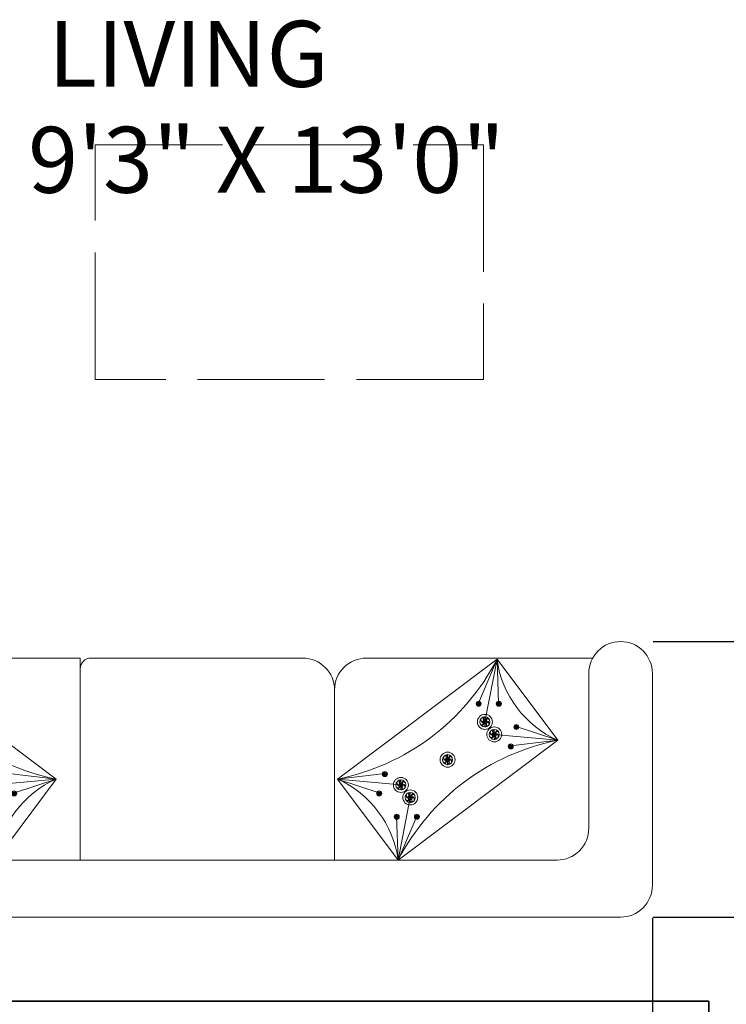
# Model space of a CAD drawing. Units: inches. Extents: x -61 to 1599, y -1316 to 257.
# Tile 165 of 204: x 1148 to 1214, y -939 to -847. Entities that reach past the tile are written whole.
import ezdxf

# ---------------------------------------------------------------- set-up
doc = ezdxf.new("R2010")
doc.units = ezdxf.units.IN
doc.header["$MEASUREMENT"] = 0
doc.linetypes.add('ACAD_ISO02W100', pattern=[15, 12, -3])
for name, color, linetype, lineweight in [('A-ANNO-DIMS', 2, 'Continuous', 18), ('A-AREA-IDEN', 1, 'Continuous', 18), ('A-FURN-LOW', 83, 'ACAD_ISO02W100', 18), ('FURNITURE', 83, 'Continuous', 18), ('WALLS', 4, 'Continuous', 35)]:
    doc.layers.add(name, color=color, linetype=linetype, lineweight=lineweight)
doc.layers.add('FUR', color=83, linetype='Continuous')
doc.styles.get("Standard").update_dxf_attribs({"font": 'arial.ttf'})
doc.dimstyles.get("Standard").update_dxf_attribs({"dimtxt": 0.18, "dimasz": 0.18, "dimexe": 0.18, "dimexo": 0.0625, "dimgap": 0.09, "dimtad": 0, "dimtih": 1, "dimtoh": 1, "dimdec": 0, "dimzin": 0, "dimdsep": 46, "dimlunit": 3, "dimtxsty": 'Standard', "dimcen": 0.09, "dimadec": 0, "dimazin": 0, "dimtfac": 1, "dimtdec": 0, "dimtofl": 0, "dimtmove": 0, "dimatfit": 3, "dimfxl": 1, "dimtolj": 1, "dimtzin": 0, "dimarcsym": 0})

# ---------------------------------------------------------------- blocks, each defined once
blk = doc.blocks.new('*U514')
at = {"layer": 'FUR'}
blk.add_open_spline([(0.005, 0.08), (-0.03, 0.048), (-0.098, -0.015), (0.075, -0.018), (0.024, -0.063), (0.005, -0.08)], degree=3, knots=[0, 0, 0, 0, 0.0954578, 0.1898773, 0.2470677, 0.2470677, 0.2470677, 0.2470677], dxfattribs=at)
blk = doc.blocks.new('*U515')
at = {"layer": 'FUR', "transparency": 16777216}
for p, rotation in [((222.173, -79.977), 60), ((222.312, -79.968), 300), ((222.178, -80.056), 120), ((222.25, -80.092), 180), ((222.317, -80.048), 240)]:
    blk.add_blockref('*U514', p, dxfattribs=dict(at, rotation=rotation))
blk.add_blockref('*U514', (222.24, -79.932), dxfattribs=at)
blk = doc.blocks.new('*U516')
at = {"layer": 'FUR'}
blk.add_open_spline([(0.005, 0.08), (-0.03, 0.048), (-0.098, -0.015), (0.075, -0.018), (0.024, -0.063), (0.005, -0.08)], degree=3, knots=[0, 0, 0, 0, 0.0954578, 0.1898773, 0.2470677, 0.2470677, 0.2470677, 0.2470677], dxfattribs=at)
blk = doc.blocks.new('*U517')
at = {"layer": 'FUR', "transparency": 16777216}
for p, rotation in [((222.173, -79.977), 60), ((222.312, -79.968), 300), ((222.178, -80.056), 120), ((222.25, -80.092), 180), ((222.317, -80.048), 240)]:
    blk.add_blockref('*U516', p, dxfattribs=dict(at, rotation=rotation))
blk.add_blockref('*U516', (222.24, -79.932), dxfattribs=at)
blk = doc.blocks.new('*U510')
at = {"layer": 'FUR'}
blk.add_open_spline([(0.005, 0.08), (-0.03, 0.048), (-0.098, -0.015), (0.075, -0.018), (0.024, -0.063), (0.005, -0.08)], degree=3, knots=[0, 0, 0, 0, 0.0954578, 0.1898773, 0.2470677, 0.2470677, 0.2470677, 0.2470677], dxfattribs=at)
blk = doc.blocks.new('*U511')
at = {"layer": 'FUR', "transparency": 16777216}
for p, rotation in [((222.173, -79.977), 60), ((222.312, -79.968), 300), ((222.178, -80.056), 120), ((222.25, -80.092), 180), ((222.317, -80.048), 240)]:
    blk.add_blockref('*U510', p, dxfattribs=dict(at, rotation=rotation))
blk.add_blockref('*U510', (222.24, -79.932), dxfattribs=at)
blk = doc.blocks.new('*U479')
at = {"layer": 'FUR'}
blk.add_open_spline([(0.015, 0.238), (-0.088, 0.143), (-0.292, -0.045), (0.224, -0.053), (0.072, -0.187), (0.015, -0.238)], degree=3, knots=[0, 0, 0, 0, 0.2846533, 0.5662105, 0.736751, 0.736751, 0.736751, 0.736751], dxfattribs=at)
blk = doc.blocks.new('*U480')
at = {"layer": 'FUR', "transparency": 16777216}
for p, rotation in [((662.517, -238.489), 60), ((662.531, -238.727), 120), ((662.745, -238.833), 180), ((662.929, -238.463), 300), ((662.944, -238.702), 240)]:
    blk.add_blockref('*U479', p, dxfattribs=dict(at, rotation=rotation))
blk.add_blockref('*U479', (662.716, -238.357), dxfattribs=at)
blk = doc.blocks.new('*U512')
at = {"layer": 'FUR'}
blk.add_open_spline([(0.005, 0.08), (-0.03, 0.048), (-0.098, -0.015), (0.075, -0.018), (0.024, -0.063), (0.005, -0.08)], degree=3, knots=[0, 0, 0, 0, 0.0954578, 0.1898773, 0.2470677, 0.2470677, 0.2470677, 0.2470677], dxfattribs=at)
blk = doc.blocks.new('*U513')
at = {"layer": 'FUR', "transparency": 16777216}
for p, rotation in [((222.173, -79.977), 60), ((222.312, -79.968), 300), ((222.178, -80.056), 120), ((222.25, -80.092), 180), ((222.317, -80.048), 240)]:
    blk.add_blockref('*U512', p, dxfattribs=dict(at, rotation=rotation))
blk.add_blockref('*U512', (222.24, -79.932), dxfattribs=at)
blk = doc.blocks.new('*U483')
at = {"layer": 'FUR'}
blk.add_open_spline([(0.015, 0.238), (-0.088, 0.143), (-0.292, -0.045), (0.224, -0.053), (0.072, -0.187), (0.015, -0.238)], degree=3, knots=[0, 0, 0, 0, 0.2846533, 0.5662105, 0.736751, 0.736751, 0.736751, 0.736751], dxfattribs=at)
blk = doc.blocks.new('*U484')
at = {"layer": 'FUR', "transparency": 16777216}
for p, rotation in [((662.517, -238.489), 60), ((662.531, -238.727), 120), ((662.745, -238.833), 180), ((662.929, -238.463), 300), ((662.944, -238.702), 240)]:
    blk.add_blockref('*U483', p, dxfattribs=dict(at, rotation=rotation))
blk.add_blockref('*U483', (662.716, -238.357), dxfattribs=at)
blk = doc.blocks.new('*U498')
at = {"layer": 'FUR'}
blk.add_open_spline([(0.005, 0.08), (-0.03, 0.048), (-0.098, -0.015), (0.075, -0.018), (0.024, -0.063), (0.005, -0.08)], degree=3, knots=[0, 0, 0, 0, 0.0954578, 0.1898773, 0.2470677, 0.2470677, 0.2470677, 0.2470677], dxfattribs=at)
blk = doc.blocks.new('*U499')
at = {"layer": 'FUR', "transparency": 16777216}
for p, rotation in [((222.173, -79.977), 60), ((222.312, -79.968), 300), ((222.178, -80.056), 120), ((222.25, -80.092), 180), ((222.317, -80.048), 240)]:
    blk.add_blockref('*U498', p, dxfattribs=dict(at, rotation=rotation))
blk.add_blockref('*U498', (222.24, -79.932), dxfattribs=at)
blk = doc.blocks.new('*U485')
at = {"layer": 'FUR'}
blk.add_open_spline([(0.015, 0.238), (-0.088, 0.143), (-0.292, -0.045), (0.224, -0.053), (0.072, -0.187), (0.015, -0.238)], degree=3, knots=[0, 0, 0, 0, 0.2846533, 0.5662105, 0.736751, 0.736751, 0.736751, 0.736751], dxfattribs=at)
blk = doc.blocks.new('*U497')
at = {"layer": 'FUR', "transparency": 16777216}
for p, rotation in [((662.517, -238.489), 60), ((662.531, -238.727), 120), ((662.745, -238.833), 180), ((662.929, -238.463), 300), ((662.944, -238.702), 240)]:
    blk.add_blockref('*U485', p, dxfattribs=dict(at, rotation=rotation))
blk.add_blockref('*U485', (662.716, -238.357), dxfattribs=at)
blk = doc.blocks.new('*U481')
at = {"layer": 'FUR'}
blk.add_open_spline([(0.015, 0.238), (-0.088, 0.143), (-0.292, -0.045), (0.224, -0.053), (0.072, -0.187), (0.015, -0.238)], degree=3, knots=[0, 0, 0, 0, 0.2846533, 0.5662105, 0.736751, 0.736751, 0.736751, 0.736751], dxfattribs=at)
blk = doc.blocks.new('*U482')
at = {"layer": 'FUR', "transparency": 16777216}
for p, rotation in [((662.517, -238.489), 60), ((662.531, -238.727), 120), ((662.745, -238.833), 180), ((662.929, -238.463), 300), ((662.944, -238.702), 240)]:
    blk.add_blockref('*U481', p, dxfattribs=dict(at, rotation=rotation))
blk.add_blockref('*U481', (662.716, -238.357), dxfattribs=at)
blk = doc.blocks.new('*U477')
at = {"layer": 'FUR'}
blk.add_open_spline([(0.005, 0.08), (-0.03, 0.048), (-0.098, -0.015), (0.075, -0.018), (0.024, -0.063), (0.005, -0.08)], degree=3, knots=[0, 0, 0, 0, 0.0954578, 0.1898773, 0.2470677, 0.2470677, 0.2470677, 0.2470677], dxfattribs=at)
blk = doc.blocks.new('*U478')
at = {"layer": 'FUR', "transparency": 16777216}
for p, rotation in [((222.173, -79.977), 60), ((222.312, -79.968), 300), ((222.178, -80.056), 120), ((222.25, -80.092), 180), ((222.317, -80.048), 240)]:
    blk.add_blockref('*U477', p, dxfattribs=dict(at, rotation=rotation))
blk.add_blockref('*U477', (222.24, -79.932), dxfattribs=at)
blk = doc.blocks.new('*U508')
at = {"layer": 'FUR'}
blk.add_open_spline([(0.005, 0.08), (-0.03, 0.048), (-0.098, -0.015), (0.075, -0.018), (0.024, -0.063), (0.005, -0.08)], degree=3, knots=[0, 0, 0, 0, 0.0954578, 0.1898773, 0.2470677, 0.2470677, 0.2470677, 0.2470677], dxfattribs=at)
blk = doc.blocks.new('*U509')
at = {"layer": 'FUR', "transparency": 16777216}
for p, rotation in [((222.173, -79.977), 60), ((222.312, -79.968), 300), ((222.178, -80.056), 120), ((222.25, -80.092), 180), ((222.317, -80.048), 240)]:
    blk.add_blockref('*U508', p, dxfattribs=dict(at, rotation=rotation))
blk.add_blockref('*U508', (222.24, -79.932), dxfattribs=at)
blk = doc.blocks.new('*U506')
at = {"layer": 'FUR'}
blk.add_open_spline([(0.005, 0.08), (-0.03, 0.048), (-0.098, -0.015), (0.075, -0.018), (0.024, -0.063), (0.005, -0.08)], degree=3, knots=[0, 0, 0, 0, 0.0954578, 0.1898773, 0.2470677, 0.2470677, 0.2470677, 0.2470677], dxfattribs=at)
blk = doc.blocks.new('*U507')
at = {"layer": 'FUR', "transparency": 16777216}
for p, rotation in [((222.173, -79.977), 60), ((222.312, -79.968), 300), ((222.178, -80.056), 120), ((222.25, -80.092), 180), ((222.317, -80.048), 240)]:
    blk.add_blockref('*U506', p, dxfattribs=dict(at, rotation=rotation))
blk.add_blockref('*U506', (222.24, -79.932), dxfattribs=at)
blk = doc.blocks.new('*U476')
at = {"layer": 'FUR'}
blk.add_open_spline([(0.005, 0.08), (-0.03, 0.048), (-0.098, -0.015), (0.075, -0.018), (0.024, -0.063), (0.005, -0.08)], degree=3, knots=[0, 0, 0, 0, 0.0954578, 0.1898773, 0.2470677, 0.2470677, 0.2470677, 0.2470677], dxfattribs=at)
blk = doc.blocks.new('*U489')
at = {"layer": 'FUR', "transparency": 16777216}
for p, rotation in [((222.173, -79.977), 60), ((222.312, -79.968), 300), ((222.178, -80.056), 120), ((222.25, -80.092), 180), ((222.317, -80.048), 240)]:
    blk.add_blockref('*U476', p, dxfattribs=dict(at, rotation=rotation))
blk.add_blockref('*U476', (222.24, -79.932), dxfattribs=at)
blk = doc.blocks.new('*U490')
at = {"layer": 'FUR'}
blk.add_open_spline([(0.005, 0.08), (-0.03, 0.048), (-0.098, -0.015), (0.075, -0.018), (0.024, -0.063), (0.005, -0.08)], degree=3, knots=[0, 0, 0, 0, 0.0954578, 0.1898773, 0.2470677, 0.2470677, 0.2470677, 0.2470677], dxfattribs=at)
blk = doc.blocks.new('*U491')
at = {"layer": 'FUR', "transparency": 16777216}
for p, rotation in [((222.173, -79.977), 60), ((222.312, -79.968), 300), ((222.178, -80.056), 120), ((222.25, -80.092), 180), ((222.317, -80.048), 240)]:
    blk.add_blockref('*U490', p, dxfattribs=dict(at, rotation=rotation))
blk.add_blockref('*U490', (222.24, -79.932), dxfattribs=at)
blk = doc.blocks.new('*U474')
at = {"layer": 'FUR'}
blk.add_open_spline([(0.005, 0.08), (-0.03, 0.048), (-0.098, -0.015), (0.075, -0.018), (0.024, -0.063), (0.005, -0.08)], degree=3, knots=[0, 0, 0, 0, 0.0954578, 0.1898773, 0.2470677, 0.2470677, 0.2470677, 0.2470677], dxfattribs=at)
blk = doc.blocks.new('*U475')
at = {"layer": 'FUR', "transparency": 16777216}
for p, rotation in [((222.173, -79.977), 60), ((222.312, -79.968), 300), ((222.178, -80.056), 120), ((222.25, -80.092), 180), ((222.317, -80.048), 240)]:
    blk.add_blockref('*U474', p, dxfattribs=dict(at, rotation=rotation))
blk.add_blockref('*U474', (222.24, -79.932), dxfattribs=at)
blk = doc.blocks.new('*U504')
at = {"layer": 'FUR'}
blk.add_open_spline([(0.015, 0.238), (-0.088, 0.143), (-0.292, -0.045), (0.224, -0.053), (0.072, -0.187), (0.015, -0.238)], degree=3, knots=[0, 0, 0, 0, 0.2846533, 0.5662105, 0.736751, 0.736751, 0.736751, 0.736751], dxfattribs=at)
blk = doc.blocks.new('*U505')
at = {"layer": 'FUR', "transparency": 16777216}
for p, rotation in [((662.517, -238.489), 60), ((662.531, -238.727), 120), ((662.745, -238.833), 180), ((662.929, -238.463), 300), ((662.944, -238.702), 240)]:
    blk.add_blockref('*U504', p, dxfattribs=dict(at, rotation=rotation))
blk.add_blockref('*U504', (662.716, -238.357), dxfattribs=at)
blk = doc.blocks.new('*U520')
at = {"layer": 'FUR'}
blk.add_open_spline([(0.015, 0.238), (-0.088, 0.143), (-0.292, -0.045), (0.224, -0.053), (0.072, -0.187), (0.015, -0.238)], degree=3, knots=[0, 0, 0, 0, 0.2846533, 0.5662105, 0.736751, 0.736751, 0.736751, 0.736751], dxfattribs=at)
blk = doc.blocks.new('*U471')
at = {"layer": 'FUR', "transparency": 16777216}
for p, rotation in [((662.517, -238.489), 60), ((662.531, -238.727), 120), ((662.745, -238.833), 180), ((662.929, -238.463), 300), ((662.944, -238.702), 240)]:
    blk.add_blockref('*U520', p, dxfattribs=dict(at, rotation=rotation))
blk.add_blockref('*U520', (662.716, -238.357), dxfattribs=at)
blk = doc.blocks.new('*U472')
at = {"layer": 'FUR'}
blk.add_open_spline([(0.005, 0.08), (-0.03, 0.048), (-0.098, -0.015), (0.075, -0.018), (0.024, -0.063), (0.005, -0.08)], degree=3, knots=[0, 0, 0, 0, 0.0954578, 0.1898773, 0.2470677, 0.2470677, 0.2470677, 0.2470677], dxfattribs=at)
blk = doc.blocks.new('*U473')
at = {"layer": 'FUR', "transparency": 16777216}
for p, rotation in [((222.173, -79.977), 60), ((222.312, -79.968), 300), ((222.178, -80.056), 120), ((222.25, -80.092), 180), ((222.317, -80.048), 240)]:
    blk.add_blockref('*U472', p, dxfattribs=dict(at, rotation=rotation))
blk.add_blockref('*U472', (222.24, -79.932), dxfattribs=at)
blk = doc.blocks.new('*U518')
at = {"layer": 'FUR'}
blk.add_open_spline([(0.015, 0.238), (-0.088, 0.143), (-0.292, -0.045), (0.224, -0.053), (0.072, -0.187), (0.015, -0.238)], degree=3, knots=[0, 0, 0, 0, 0.2846533, 0.5662105, 0.736751, 0.736751, 0.736751, 0.736751], dxfattribs=at)
blk = doc.blocks.new('*U519')
at = {"layer": 'FUR', "transparency": 16777216}
for p, rotation in [((662.517, -238.489), 60), ((662.531, -238.727), 120), ((662.745, -238.833), 180), ((662.929, -238.463), 300), ((662.944, -238.702), 240)]:
    blk.add_blockref('*U518', p, dxfattribs=dict(at, rotation=rotation))
blk.add_blockref('*U518', (662.716, -238.357), dxfattribs=at)
blk = doc.blocks.new('*U494')
at = {"layer": 'FUR'}
blk.add_open_spline([(0.005, 0.08), (-0.03, 0.048), (-0.098, -0.015), (0.075, -0.018), (0.024, -0.063), (0.005, -0.08)], degree=3, knots=[0, 0, 0, 0, 0.0954578, 0.1898773, 0.2470677, 0.2470677, 0.2470677, 0.2470677], dxfattribs=at)
blk = doc.blocks.new('*U495')
at = {"layer": 'FUR', "transparency": 16777216}
for p, rotation in [((222.173, -79.977), 60), ((222.312, -79.968), 300), ((222.178, -80.056), 120), ((222.25, -80.092), 180), ((222.317, -80.048), 240)]:
    blk.add_blockref('*U494', p, dxfattribs=dict(at, rotation=rotation))
blk.add_blockref('*U494', (222.24, -79.932), dxfattribs=at)
blk = doc.blocks.new('*U502')
at = {"layer": 'FUR'}
blk.add_open_spline([(0.015, 0.238), (-0.088, 0.143), (-0.292, -0.045), (0.224, -0.053), (0.072, -0.187), (0.015, -0.238)], degree=3, knots=[0, 0, 0, 0, 0.2846533, 0.5662105, 0.736751, 0.736751, 0.736751, 0.736751], dxfattribs=at)
blk = doc.blocks.new('*U503')
at = {"layer": 'FUR', "transparency": 16777216}
for p, rotation in [((662.517, -238.489), 60), ((662.531, -238.727), 120), ((662.745, -238.833), 180), ((662.929, -238.463), 300), ((662.944, -238.702), 240)]:
    blk.add_blockref('*U502', p, dxfattribs=dict(at, rotation=rotation))
blk.add_blockref('*U502', (662.716, -238.357), dxfattribs=at)
blk = doc.blocks.new('*U486')
at = {"layer": 'FUR'}
blk.add_open_spline([(0.015, 0.238), (-0.088, 0.143), (-0.292, -0.045), (0.224, -0.053), (0.072, -0.187), (0.015, -0.238)], degree=3, knots=[0, 0, 0, 0, 0.2846533, 0.5662105, 0.736751, 0.736751, 0.736751, 0.736751], dxfattribs=at)
blk = doc.blocks.new('*U487')
at = {"layer": 'FUR', "transparency": 16777216}
for p, rotation in [((662.517, -238.489), 60), ((662.531, -238.727), 120), ((662.745, -238.833), 180), ((662.929, -238.463), 300), ((662.944, -238.702), 240)]:
    blk.add_blockref('*U486', p, dxfattribs=dict(at, rotation=rotation))
blk.add_blockref('*U486', (662.716, -238.357), dxfattribs=at)
blk = doc.blocks.new('*U492')
at = {"layer": 'FUR'}
blk.add_open_spline([(0.005, 0.08), (-0.03, 0.048), (-0.098, -0.015), (0.075, -0.018), (0.024, -0.063), (0.005, -0.08)], degree=3, knots=[0, 0, 0, 0, 0.0954578, 0.1898773, 0.2470677, 0.2470677, 0.2470677, 0.2470677], dxfattribs=at)
blk = doc.blocks.new('*U493')
at = {"layer": 'FUR', "transparency": 16777216}
for p, rotation in [((222.173, -79.977), 60), ((222.312, -79.968), 300), ((222.178, -80.056), 120), ((222.25, -80.092), 180), ((222.317, -80.048), 240)]:
    blk.add_blockref('*U492', p, dxfattribs=dict(at, rotation=rotation))
blk.add_blockref('*U492', (222.24, -79.932), dxfattribs=at)
blk = doc.blocks.new('*U500')
at = {"layer": 'FUR'}
blk.add_open_spline([(0.005, 0.08), (-0.03, 0.048), (-0.098, -0.015), (0.075, -0.018), (0.024, -0.063), (0.005, -0.08)], degree=3, knots=[0, 0, 0, 0, 0.0954578, 0.1898773, 0.2470677, 0.2470677, 0.2470677, 0.2470677], dxfattribs=at)
blk = doc.blocks.new('*U501')
at = {"layer": 'FUR', "transparency": 16777216}
for p, rotation in [((222.173, -79.977), 60), ((222.312, -79.968), 300), ((222.178, -80.056), 120), ((222.25, -80.092), 180), ((222.317, -80.048), 240)]:
    blk.add_blockref('*U500', p, dxfattribs=dict(at, rotation=rotation))
blk.add_blockref('*U500', (222.24, -79.932), dxfattribs=at)
blk = doc.blocks.new('*U496')
at = {"layer": 'FUR'}
blk.add_open_spline([(0.005, 0.08), (-0.03, 0.048), (-0.098, -0.015), (0.075, -0.018), (0.024, -0.063), (0.005, -0.08)], degree=3, knots=[0, 0, 0, 0, 0.0954578, 0.1898773, 0.2470677, 0.2470677, 0.2470677, 0.2470677], dxfattribs=at)
blk = doc.blocks.new('*U488')
at = {"layer": 'FUR', "transparency": 16777216}
for p, rotation in [((222.173, -79.977), 60), ((222.312, -79.968), 300), ((222.178, -80.056), 120), ((222.25, -80.092), 180), ((222.317, -80.048), 240)]:
    blk.add_blockref('*U496', p, dxfattribs=dict(at, rotation=rotation))
blk.add_blockref('*U496', (222.24, -79.932), dxfattribs=at)
blk = doc.blocks.new('SOFA-THREE-SEAT-ALT-2')
for p, q in [((30, 24.442), (6.996, 24.38)), ((12.664, 24.333), (12.509, 20.191)), ((12.664, 24.333), (13.805, 18.423)), ((12.664, 24.333), (14.414, 20.191)), ((30, 23.442), (29.997, 24.442)), ((51, 24.442), (31, 24.442)), ((78.369, 24.442), (57, 24.442)), ((69.336, 24.333), (67.586, 20.191)), ((69.336, 24.333), (68.194, 18.423)), ((69.336, 24.333), (69.49, 20.191)), ((6, 23), (5.999, 23.377)), ((30, 23.442), (30, 5.382)), ((54, 21.442), (54, 5.382)), ((54, 21.442), (54, 21.442)), ((12.49, 20.139), (12.49, 20.299)), ((12.49, 20.139), (12.49, 19.979)), ((14.394, 20.139), (14.394, 20.299)), ((14.394, 20.139), (14.394, 19.979)), ((67.605, 20.139), (67.605, 20.299)), ((67.605, 20.139), (67.605, 19.979)), ((69.509, 20.139), (69.509, 20.299)), ((69.509, 20.139), (69.509, 19.979)), ((13.805, 18.423), (13.805, 18.899)), ((68.194, 18.423), (68.194, 18.899)), ((6.926, 16.687), (10.859, 17.993)), ((10.84, 17.94), (10.84, 18.1)), ((10.84, 17.94), (10.84, 17.78)), ((13.805, 18.423), (13.805, 17.946)), ((68.194, 18.423), (68.194, 17.946)), ((69.079, 17.243), (69.079, 17.719)), ((75.074, 16.687), (71.14, 17.993)), ((71.159, 17.94), (71.159, 18.1)), ((71.159, 17.94), (71.159, 17.78)), ((6.926, 16.687), (12.92, 17.243)), ((75.074, 16.687), (69.079, 17.243)), ((69.079, 17.243), (69.079, 16.766)), ((6.926, 16.687), (11.391, 16.164)), ((11.372, 16.112), (11.372, 16.272)), ((11.372, 16.112), (11.372, 15.952)), ((75.074, 16.687), (70.608, 16.164)), ((70.627, 16.112), (70.627, 16.272)), ((70.627, 16.112), (70.627, 15.952)), ((17.327, 14.857), (17.327, 15.334)), ((64.672, 14.857), (64.672, 15.334)), ((17.327, 14.857), (17.327, 14.381)), ((64.672, 14.857), (64.672, 14.381)), ((27.729, 13.028), (21.735, 12.472)), ((23.243, 13.498), (23.243, 13.658)), ((23.243, 13.498), (23.243, 13.338)), ((27.729, 13.028), (23.263, 13.551)), ((27.729, 13.028), (23.795, 11.722)), ((54.271, 13.028), (58.736, 13.551)), ((54.271, 13.028), (60.265, 12.472)), ((54.271, 13.028), (58.204, 11.722)), ((58.756, 13.498), (58.756, 13.658)), ((58.756, 13.498), (58.756, 13.338)), ((21.735, 12.472), (21.735, 12.948)), ((21.735, 12.472), (21.735, 11.995)), ((60.265, 12.472), (60.265, 12.948)), ((60.265, 12.472), (60.265, 11.995)), ((20.849, 11.292), (20.849, 11.769)), ((21.991, 5.382), (20.849, 11.292)), ((20.849, 11.292), (20.849, 10.816)), ((23.776, 11.67), (23.776, 11.83)), ((23.776, 11.67), (23.776, 11.51)), ((58.224, 11.67), (58.224, 11.83)), ((58.224, 11.67), (58.224, 11.51)), ((60.009, 5.382), (61.15, 11.292)), ((61.15, 11.292), (61.15, 11.769)), ((61.15, 11.292), (61.15, 10.816)), ((20.221, 9.471), (20.221, 9.631)), ((20.221, 9.471), (20.221, 9.311)), ((21.991, 5.382), (20.241, 9.523)), ((21.991, 5.382), (22.145, 9.523)), ((22.125, 9.471), (22.125, 9.631)), ((22.125, 9.471), (22.125, 9.311)), ((60.009, 5.382), (59.854, 9.523)), ((59.874, 9.471), (59.874, 9.631)), ((59.874, 9.471), (59.874, 9.311)), ((60.009, 5.382), (61.759, 9.523)), ((61.778, 9.471), (61.778, 9.631)), ((61.778, 9.471), (61.778, 9.311))]:
    blk.add_line(p, q)
blk.add_lwpolyline([(78, 8.382), (78, 23, -0.414214), (81, 26), (81, 26, -0.414214), (84, 23), (84, 3, -0.414214), (81, 0), (3, 0, -0.414214), (0, 3), (0, 23, -0.414214), (3, 26), (3, 26, -0.414214), (6, 23), (6, 8.382, 0.414214), (9, 5.382), (75, 5.382, 0.414214)], format="xyb", close=True)
for points in [[(27.729, 13.028), (12.664, 24.333), (6.926, 16.687), (21.991, 5.382)], [(54.271, 13.028), (69.336, 24.333), (75.074, 16.687), (60.009, 5.382)]]:
    blk.add_lwpolyline(points, close=True)
for centre, radius in [((12.49, 20.139), 0.238), ((12.49, 20.139), 0.16), ((14.394, 20.139), 0.238), ((14.394, 20.139), 0.16), ((67.605, 20.139), 0.238), ((67.605, 20.139), 0.16), ((69.509, 20.139), 0.238), ((69.509, 20.139), 0.16), ((13.805, 18.423), 0.71), ((13.805, 18.423), 0.476), ((68.194, 18.423), 0.71), ((68.194, 18.423), 0.476), ((10.84, 17.94), 0.238), ((10.84, 17.94), 0.16), ((69.079, 17.243), 0.71), ((69.079, 17.243), 0.476), ((71.159, 17.94), 0.238), ((71.159, 17.94), 0.16), ((11.372, 16.112), 0.238), ((11.372, 16.112), 0.16), ((70.627, 16.112), 0.238), ((70.627, 16.112), 0.16), ((17.327, 14.857), 0.71), ((17.327, 14.857), 0.476), ((64.672, 14.857), 0.71), ((64.672, 14.857), 0.476), ((21.735, 12.472), 0.71), ((23.243, 13.498), 0.238), ((23.243, 13.498), 0.16), ((58.756, 13.498), 0.238), ((58.756, 13.498), 0.16), ((60.265, 12.472), 0.71), ((21.735, 12.472), 0.476), ((60.265, 12.472), 0.476), ((20.849, 11.292), 0.71), ((20.849, 11.292), 0.476), ((23.776, 11.67), 0.238), ((23.776, 11.67), 0.16), ((58.224, 11.67), 0.238), ((58.224, 11.67), 0.16), ((61.15, 11.292), 0.71), ((61.15, 11.292), 0.476), ((20.221, 9.471), 0.238), ((20.221, 9.471), 0.16), ((22.125, 9.471), 0.238), ((22.125, 9.471), 0.16), ((59.874, 9.471), 0.238), ((59.874, 9.471), 0.16), ((61.778, 9.471), 0.238), ((61.778, 9.471), 0.16)]:
    blk.add_circle(centre, radius)
for centre, radius, start, end in [((6.999, 23.38), 1, 90.15417, 180.15417), ((2.937, 25.656), 9.816, 293.97422, 352.25297), ((31.951, 34.344), 21.731, 207.43163, 258.79556), ((31, 23.442), 1, 89.99998, 179.99998), ((51, 21.442), 3, 359.99998, 89.99998), ((57, 21.442), 3, 90, 180.00002), ((50.048, 34.344), 21.731, 281.20444, 332.56837), ((79.062, 25.656), 9.816, 187.74703, 246.02578), ((2.703, -4.63), 21.731, 27.43163, 78.79556), ((79.296, -4.63), 21.731, 101.20444, 152.56837), ((31.717, 4.058), 9.816, 113.97422, 172.25297), ((50.282, 4.058), 9.816, 7.74703, 66.02578)]:
    blk.add_arc(centre, radius, start, end)
at = {"xscale": -1, "rotation": 180}
for name, p in [('*U511', (-209.755, -59.873)), ('*U513', (-207.851, -59.873)), ('*U480', (-648.925, -220.173)), ('*U515', (-211.405, -62.072)), ('*U517', (-210.873, -63.901)), ('*U484', (-645.403, -223.738)), ('*U509', (-199.001, -66.514)), ('*U482', (-640.996, -226.123)), ('*U497', (-641.881, -227.303)), ('*U507', (-198.469, -68.343)), ('*U499', (-202.024, -70.541)), ('*U478', (-200.12, -70.541))]:
    blk.add_blockref(name, p, dxfattribs=at)
at = {"rotation": 180}
for name, p in [('*U495', (289.85, -59.873)), ('*U493', (291.754, -59.873)), ('*U503', (730.924, -220.173)), ('*U487', (731.81, -221.352)), ('*U488', (293.404, -62.072)), ('*U501', (292.872, -63.901)), ('*U519', (727.402, -223.738)), ('*U491', (281.001, -66.514)), ('*U505', (722.995, -226.123)), ('*U489', (280.469, -68.343)), ('*U471', (723.88, -227.303)), ('*U475', (282.119, -70.541)), ('*U473', (284.023, -70.541))]:
    blk.add_blockref(name, p, dxfattribs=at)
blk = doc.blocks.new('*D684')
at = {"layer": 'A-ANNO-DIMS', "color": 0, "lineweight": -2, "transparency": 16777216}
for p, q in [((1123.375, -931.288), (1123.375, -944.005)), ((1207.375, -931.288), (1207.375, -944.005)), ((1123.555, -943.825), (1164.47, -943.825)), ((1207.195, -943.825), (1166.279, -943.825))]:
    blk.add_line(p, q, dxfattribs=at)
at = {"layer": 'A-ANNO-DIMS', "color": 0, "transparency": 16777216}
for points in [[(1123.555, -943.795), (1123.555, -943.855), (1123.375, -943.825)], [(1207.195, -943.795), (1207.195, -943.855), (1207.375, -943.825)]]:
    blk.add_solid(points, dxfattribs=at)
at = {"layer": 'DEFPOINTS', "color": 0, "transparency": 16777216}
for p in [(1123.375, -931.225), (1207.375, -931.225), (1207.375, -943.825)]:
    blk.add_point(p, dxfattribs=at)
at = {"layer": 'A-ANNO-DIMS', "color": 0, "transparency": 16777216, "insert": (1165.375, -943.825), "char_height": 0.18, "attachment_point": 5}
blk.add_mtext('\\A1;SOFA 84 TYP.', dxfattribs=at)
blk = doc.blocks.new('*D685')
at = {"layer": 'A-ANNO-DIMS', "color": 0, "lineweight": -2, "transparency": 16777216}
for p, q in [((1207.437, -905.225), (1220.155, -905.225)), ((1219.975, -905.405), (1219.975, -918.043)), ((1219.975, -931.045), (1219.975, -918.407)), ((1207.437, -931.225), (1220.155, -931.225))]:
    blk.add_line(p, q, dxfattribs=at)
at = {"layer": 'A-ANNO-DIMS', "color": 0, "transparency": 16777216}
for points in [[(1219.945, -905.405), (1220.005, -905.405), (1219.975, -905.225)], [(1219.945, -931.045), (1220.005, -931.045), (1219.975, -931.225)]]:
    blk.add_solid(points, dxfattribs=at)
at = {"layer": 'DEFPOINTS', "color": 0, "transparency": 16777216}
for p in [(1207.375, -905.225), (1219.975, -905.225), (1207.375, -931.225)]:
    blk.add_point(p, dxfattribs=at)
at = {"layer": 'A-ANNO-DIMS', "color": 0, "transparency": 16777216, "insert": (1219.975, -918.225), "char_height": 0.18, "attachment_point": 5}
blk.add_mtext('\\A1;26 TYP.', dxfattribs=at)

msp = doc.modelspace()

# ---------------------------------------------------------------- linework, layer by layer
at = {"layer": 'A-FURN-LOW'}
msp.add_lwpolyline([(1191.4399, -880.5045), (1154.794, -880.5045), (1154.794, -858.3381), (1191.4399, -858.3381)], close=True, dxfattribs=at)
at = {"layer": 'WALLS'}
for p in [(1097.7028, -939.169), (1212.7028, -1052.169)]:
    msp.add_line(p, (1212.7028, -939.169), dxfattribs=at)

# ---------------------------------------------------------------- block references
at = {"layer": 'FURNITURE'}
msp.add_blockref('SOFA-THREE-SEAT-ALT-2', (1123.375, -931.225), dxfattribs=at)

# ---------------------------------------------------------------- texts
at = {"layer": 'A-AREA-IDEN'}
for s, height, p in [('   LIVING', 6.22364, (1144.6485, -852.8797)), ('  9\'3" X 13\'0"', 6.223643, (1144.6485, -862.8775))]:
    msp.add_text(s, height=height, dxfattribs=at).set_placement(p)

# ---------------------------------------------------------------- dimensions: what is measured, and where the dimension line sits
at = {"layer": 'A-ANNO-DIMS'}
dim = msp.add_linear_dim(base=(1219.9746, -905.2253), p1=(1207.3746, -931.2253), p2=(1207.3746, -905.2253), angle=90, text='<> TYP.', dimstyle='Standard', override={"dimdec": 0, "dimlfac": 1, "dimrnd": 0, "dimzin": 0, "dimdsep": 46, "dimlunit": 2}, dxfattribs=at)
dim.commit()
dim.dimension.update_dxf_attribs({"geometry": '*D685', "text_midpoint": (1219.9746, -918.2253)})
dim = msp.add_linear_dim(base=(1207.3746, -943.8253), p1=(1123.3746, -931.2253), p2=(1207.3746, -931.2253), text='SOFA <> TYP.', dimstyle='Standard', override={"dimdec": 0, "dimlfac": 1, "dimrnd": 0, "dimzin": 0, "dimdsep": 46, "dimlunit": 2}, dxfattribs=at)
dim.commit()
dim.dimension.update_dxf_attribs({"geometry": '*D684', "text_midpoint": (1165.3746, -943.8253)})

doc.saveas('drawing.dxf')
